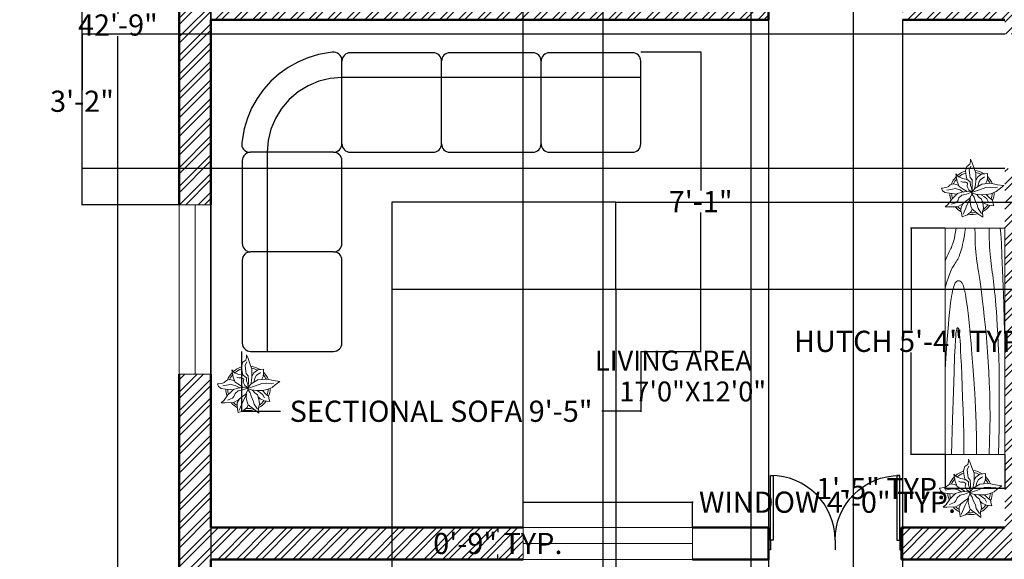
# Model space of a CAD drawing. Units: inches. Extents: x -71 to 434, y -519 to 67.
# Tile 2 of 7: x -58 to 221, y -377 to -224. Entities that reach past the tile are written whole.
import ezdxf

# ---------------------------------------------------------------- set-up
doc = ezdxf.new("R2010")
doc.units = ezdxf.units.IN
doc.header["$MEASUREMENT"] = 0
for name, color, linetype, lineweight in [('A-ANNO-DIMS', 7, 'Continuous', 18), ('A-AREA-IDEN', 7, 'Continuous', 25), ('A-WALL-PATT', 8, 'Continuous', 13), ('CAY', 94, 'Continuous', 13), ('DOOR', 3, 'Continuous', 25), ('FURNITURE', 5, 'Continuous', 18), ('WALL', 50, 'Continuous', 50), ('WINDOW', 1, 'Continuous', 18)]:
    doc.layers.add(name, color=color, linetype=linetype, lineweight=lineweight)
doc.layers.add('NOITHAT', color=21, linetype='Continuous')
doc.styles.add('ATT', font='romans.shx')
doc.styles.get("Standard").update_dxf_attribs({"font": 'arial.ttf'})
doc.dimstyles.get("Standard").update_dxf_attribs({"dimtxt": 6, "dimasz": 0.18, "dimexe": 0.18, "dimexo": 0.0625, "dimgap": 0.09, "dimtad": 0, "dimtih": 1, "dimtoh": 1, "dimdec": 0, "dimzin": 0, "dimdsep": 46, "dimlunit": 3, "dimtxsty": 'Standard', "dimcen": 0.09, "dimadec": 0, "dimazin": 0, "dimtfac": 1, "dimtdec": 0, "dimtofl": 0, "dimtmove": 0, "dimatfit": 3, "dimfxl": 1, "dimtolj": 1, "dimtzin": 0, "dimarcsym": 0})

# ---------------------------------------------------------------- blocks, each defined once
blk = doc.blocks.new('A$C74556632')
at = {"layer": 'NOITHAT'}
for p, q in [((462.2, 1788.5), (398.2, 1769.7)), ((544.2, 1802.9), (462.2, 1788.5)), ((1152.9, 1800), (652.9, 1800)), ((1752.9, 1800), (1252.9, 1800)), ((2352.9, 1800), (1852.9, 1800)), ((336.7, 1744), (278.4, 1711.6)), ((398.2, 1769.7), (336.7, 1744)), ((602.9, 1250), (602.9, 1750)), ((1202.9, 1250), (1202.9, 1750)), ((1802.9, 1250), (1802.9, 1750)), ((2402.9, 1250), (2402.9, 1750)), ((224.1, 1672.9), (174.4, 1628.5)), ((278.4, 1711.6), (224.1, 1672.9)), ((174.4, 1628.5), (130, 1578.8)), ((463.8, 1628), (398.6, 1601)), ((532.4, 1644.5), (463.8, 1628)), ((602.9, 1650), (532.4, 1644.5)), ((2402.9, 1650), (602.9, 1650)), ((130, 1578.8), (91.3, 1524.5)), ((338.3, 1564.1), (284.6, 1518.2)), ((398.6, 1601), (338.3, 1564.1)), ((91.3, 1524.5), (58.9, 1466.2)), ((284.6, 1518.2), (238.8, 1464.5)), ((58.9, 1466.2), (33.2, 1404.7)), ((238.8, 1464.5), (201.9, 1404.3)), ((33.2, 1404.7), (14.4, 1340.7)), ((201.9, 1404.3), (174.9, 1339.1)), ((14.4, 1340.7), (0, 1258.7)), ((174.9, 1339.1), (158.4, 1270.4)), ((158.4, 1270.4), (152.9, 1200)), ((552.9, 1200), (49.2, 1200)), ((152.9, 1200), (152.9, 0)), ((652.9, 1200), (1152.9, 1200)), ((677.9, 1200), (677.9, 1200)), ((1252.9, 1200), (1752.9, 1200)), ((1852.9, 1200), (2352.9, 1200)), ((2.9, 1150), (2.9, 650)), ((602.9, 650), (602.9, 1150)), ((2252.9, 900), (902.9, 900)), ((902.9, 900), (902.9, 375)), ((2252.9, 375), (2252.9, 900)), ((552.9, 600), (52.9, 600)), ((2.9, 550), (2.9, 50)), ((602.9, 50), (602.9, 550)), ((902.9, 375), (2252.9, 375)), ((52.9, 0), (552.9, 0))]:
    blk.add_line(p, q, dxfattribs=at)
for centre, start, end in [((552.9, 1753.6), 0, 99.97066), ((652.9, 1750), 90, 180), ((1152.9, 1750), 0, 90), ((1252.9, 1750), 90, 180), ((1752.9, 1750), 0, 90), ((1852.9, 1750), 90, 180), ((2352.9, 1750), 0, 90), ((49.2, 1250), 170.02934, 270), ((552.9, 1250), 270, 0), ((652.9, 1250), 180, 270), ((1152.9, 1250), 270, 0), ((1252.9, 1250), 180, 270), ((1752.9, 1250), 270, 0), ((1852.9, 1250), 180, 270), ((2352.9, 1250), 270, 0), ((52.9, 1150), 90, 180), ((552.9, 1150), 0, 90), ((52.9, 650), 180, 270), ((52.9, 550), 90, 180), ((552.9, 650), 270, 0), ((552.9, 550), 0, 90), ((52.9, 50), 180, 270), ((552.9, 50), 270, 0)]:
    blk.add_arc(centre, 50, start, end, dxfattribs=at)
blk = doc.blocks.new('*U13')
for p, q in [((0, 0), (0, -6)), ((40, 0), (40, -6))]:
    blk.add_line(p, q)
blk.add_lwpolyline([(0, 0), (0, 40), (1.75, 40), (1.75, 0)], close=True)
blk.add_arc((0, 0), 40, 0, 90)
blk = doc.blocks.new('Hutch - 19 x 72 in.')
for p, q in [((0, -19), (0, 0)), ((0, 0), (71.999994, 0)), ((71.999994, 0), (71.999994, -19)), ((71.999994, -19), (0, -19))]:
    blk.add_line(p, q)
for points in [[(26.99999, 0), (32.30411, -0.35238), (36.66731, -0.66276), (40.20336, -0.93603), (43.02603, -1.17708), (45.2491, -1.39079), (46.98632, -1.58203), (48.35147, -1.7557), (49.45833, -1.91667), (50.40388, -2.06917), (51.21809, -2.21484), (51.91414, -2.35465), (52.5052, -2.48958), (53.00447, -2.6206), (53.42512, -2.7487), (53.78035, -2.87484), (54.08333, -3), (54.34537, -3.12516), (54.57031, -3.2513), (54.76008, -3.37939), (54.91666, -3.51042), (55.04198, -3.64534), (55.13801, -3.78516), (55.2067, -3.93083), (55.24999, -4.08333), (55.26904, -4.24316), (55.26171, -4.40885), (55.22509, -4.57845), (55.15624, -4.75), (55.05224, -4.92155), (54.91015, -5.09115), (54.72704, -5.25684), (54.49999, -5.41667), (54.22493, -5.56934), (53.89322, -5.71615), (53.49511, -5.85905), (53.02083, -6), (52.4606, -6.14095), (51.80468, -6.28385), (51.04329, -6.43066), (50.16666, -6.58333), (49.16007, -6.74381), (47.98892, -6.91406), (46.61368, -7.09603), (44.99478, -7.29167), (43.09268, -7.50293), (40.86783, -7.73177), (38.28067, -7.98014), (35.29166, -8.25), (31.87654, -8.54053), (28.07226, -8.83984), (23.93107, -9.1333), (19.5052, -9.40625), (14.84692, -9.64404), (10.00846, -9.83203), (5.04207, -9.95557), (0, -10)], [(52.99999, 0), (54.87133, -0.53955), (56.39257, -1.03516), (57.61205, -1.48975), (58.57812, -1.90625), (59.3391, -2.2876), (59.94335, -2.63672), (60.4392, -2.95654), (60.87499, -3.25), (61.29247, -3.52002), (61.70702, -3.76953), (62.12743, -4.00146), (62.56249, -4.21875), (63.02099, -4.42432), (63.51171, -4.62109), (64.04345, -4.81201), (64.62499, -5), (65.26489, -5.1875), (65.9707, -5.375), (66.74975, -5.5625), (67.60937, -5.75), (68.55688, -5.9375), (69.5996, -6.125), (70.744867, -6.3125), (71.999994, -6.5)], [(61.49999, 0), (62.35961, -0.35254), (63.08007, -0.66406), (63.68627, -0.94043), (64.20312, -1.1875), (64.65551, -1.41113), (65.06835, -1.61719), (65.46655, -1.81152), (65.87499, -2), (66.31762, -2.1875), (66.81445, -2.375), (67.38452, -2.5625), (68.04687, -2.75), (68.82055, -2.9375), (69.7246, -3.125), (70.77807, -3.3125), (71.999994, -3.5)], [(0, -2), (11.2006, -2.34123), (19.90169, -2.62044), (26.43969, -2.84595), (31.15103, -3.02604), (34.37214, -3.16903), (36.43945, -3.2832), (37.68936, -3.37687), (38.45833, -3.45833), (39.02937, -3.53459), (39.472, -3.60742), (39.80232, -3.67733), (40.03645, -3.74479), (40.1905, -3.8103), (40.28059, -3.87435), (40.32283, -3.93742), (40.33333, -4), (40.32405, -4.0625), (40.29036, -4.125), (40.22346, -4.1875), (40.11458, -4.25), (39.95491, -4.3125), (39.73567, -4.375), (39.44807, -4.4375), (39.08333, -4.5), (38.62491, -4.56282), (38.02538, -4.6276), (37.22957, -4.69629), (36.18228, -4.77083), (34.82836, -4.85319), (33.11262, -4.94531), (30.97989, -5.04915), (28.37499, -5.16667), (25.27416, -5.29818), (21.77929, -5.4375), (18.02368, -5.57682), (14.14062, -5.70833), (10.26342, -5.82422), (6.52539, -5.91667), (3.05981, -5.97786), (0, -6)], [(71.999994, -9.5), (70.071934, -9.51147), (68.38801, -9.54492), (66.91113, -9.59888), (65.60416, -9.67187), (64.43001, -9.76245), (63.35156, -9.86914), (62.3317, -9.99048), (61.33333, -10.125), (60.32128, -10.27157), (59.26822, -10.43034), (58.14876, -10.60181), (56.93749, -10.78646), (55.60904, -10.98478), (54.13801, -11.19726), (52.49902, -11.4244), (50.66666, -11.66667), (48.62239, -11.92358), (46.37499, -12.19075), (43.9401, -12.46281), (41.33333, -12.73437), (38.57031, -13.00008), (35.66666, -13.25456), (32.63801, -13.49243), (29.49999, -13.70833), (26.26367, -13.89689), (22.92187, -14.05273), (19.46289, -14.17049), (15.875, -14.24479), (12.14648, -14.27026), (8.26562, -14.24154), (4.2207, -14.15324), (0, -14)], [(0, -17), (8.37556, -17.14274), (15.58268, -17.20443), (21.74194, -17.19775), (26.97395, -17.13542), (31.39933, -17.03011), (35.13866, -16.89453), (38.31257, -16.74137), (41.04166, -16.58333), (43.4322, -16.43083), (45.5332, -16.28516), (47.37931, -16.14534), (49.0052, -16.01042), (50.44555, -15.87939), (51.73502, -15.7513), (52.90828, -15.62516), (53.99999, -15.5), (55.04044, -15.37508), (56.04231, -15.25065), (57.01391, -15.1272), (57.96353, -15.00521), (58.89949, -14.88517), (59.83007, -14.76758), (60.76358, -14.65291), (61.70833, -14.54167), (62.6752, -14.43465), (63.68554, -14.33398), (64.76326, -14.24211), (65.93229, -14.16146), (67.21655, -14.09448), (68.63997, -14.04362), (70.226475, -14.01131), (71.999994, -14)], [(36.99999, -19), (42.40038, -18.8125), (47.95312, -18.625), (53.43554, -18.4375), (58.62499, -18.25), (63.29882, -18.0625), (67.23437, -17.875), (70.208978, -17.6875), (71.999994, -17.5)]]:
    blk.add_lwpolyline(points)
blk = doc.blocks.new('*D18')
at = {"layer": 'A-ANNO-DIMS', "color": 0, "lineweight": -2, "transparency": 16777216}
for p, q in [((-12.65, 30.83), (-30.15, 30.83)), ((-29.97, 30.65), (-29.97, -222.51)), ((-29.97, -481.99), (-29.97, -228.82)), ((-12.65, -482.17), (-30.15, -482.17))]:
    blk.add_line(p, q, dxfattribs=at)
at = {"layer": 'A-ANNO-DIMS', "color": 0, "transparency": 16777216}
for points in [[(-30, 30.65), (-29.94, 30.65), (-29.97, 30.83)], [(-30, -481.99), (-29.94, -481.99), (-29.97, -482.17)]]:
    blk.add_solid(points, dxfattribs=at)
at = {"layer": 'Defpoints', "color": 0, "transparency": 16777216}
for p in [(-12.59, 30.83), (-29.97, -482.17), (-12.59, -482.17)]:
    blk.add_point(p, dxfattribs=at)
at = {"layer": 'A-ANNO-DIMS', "color": 0, "transparency": 16777216, "insert": (-29.97, -225.67), "char_height": 6, "attachment_point": 5}
blk.add_mtext('\\A1;42\'-9"', dxfattribs=at)
blk = doc.blocks.new('12PPLT12')
at = {"color": 0, "linetype": 'ByBlock'}
for p, q in [((-0.05, 0.632), (-0.034, 0.694)), ((-0.034, 0.694), (-0.032, 0.751)), ((-0.032, 0.751), (-0.002, 0.689)), ((-0.002, 0.689), (0.044, 0.559)), ((-0.148, 0.486), (-0.116, 0.583)), ((-0.132, 0.367), (-0.148, 0.486)), ((-0.116, 0.583), (-0.05, 0.632)), ((-0.064, 0.51), (-0.026, 0.591)), ((-0.05, 0.38), (-0.064, 0.51)), ((0.044, 0.559), (0.09, 0.432)), ((-0.349, 0.334), (-0.362, 0.415)), ((-0.362, 0.415), (-0.303, 0.35)), ((-0.332, 0.247), (-0.349, 0.334)), ((-0.289, 0.136), (-0.332, 0.247)), ((-0.303, 0.35), (-0.208, 0.312)), ((-0.205, 0.231), (-0.251, 0.247)), ((-0.208, 0.312), (-0.105, 0.29)), ((-0.137, 0.231), (-0.205, 0.231)), ((-0.097, 0.204), (-0.137, 0.231)), ((-0.108, 0.279), (-0.132, 0.367)), ((-0.105, 0.29), (-0.037, 0.236)), ((-0.043, 0.334), (-0.05, 0.38)), ((0.003, 0.279), (-0.043, 0.334)), ((-0.037, 0.236), (-0.034, 0.158)), ((0.009, 0.169), (0.003, 0.279)), ((0.09, 0.253), (0.082, 0.174)), ((0.09, 0.432), (0.09, 0.339)), ((0.09, 0.339), (0.09, 0.253)), ((0.093, 0.282), (0.134, 0.347)), ((0.155, 0.228), (0.131, 0.13)), ((0.134, 0.347), (0.22, 0.415)), ((0.193, 0.293), (0.155, 0.228)), ((0.25, 0.328), (0.193, 0.293)), ((0.22, 0.415), (0.291, 0.421)), ((0.28, 0.353), (0.25, 0.328)), ((0.291, 0.421), (0.35, 0.429)), ((0.342, 0.266), (0.304, 0.19)), ((0.348, 0.331), (0.342, 0.266)), ((0.35, 0.429), (0.348, 0.331)), ((-0.671, 0.098), (-0.687, 0.095)), ((-0.687, 0.095), (-0.666, 0.036)), ((-0.59, 0.109), (-0.671, 0.098)), ((-0.666, 0.036), (-0.601, -0.005)), ((-0.536, 0.125), (-0.59, 0.109)), ((-0.563, 0.052), (-0.441, 0.074)), ((-0.487, 0.171), (-0.536, 0.125)), ((-0.425, 0.193), (-0.487, 0.171)), ((-0.441, 0.074), (-0.373, 0.084)), ((-0.346, 0.179), (-0.425, 0.193)), ((-0.373, 0.084), (-0.27, 0.057)), ((-0.292, 0.149), (-0.346, 0.179)), ((-0.229, 0.003), (-0.324, -0.027)), ((-0.194, 0.074), (-0.289, 0.136)), ((-0.27, 0.057), (-0.186, 0.006)), ((-0.069, 0.027), (-0.229, 0.003)), ((-0.108, 0.019), (-0.194, 0.074)), ((-0.01, 0.003), (-0.121, -0.038)), ((-0.11, 0.133), (-0.097, 0.204)), ((-0.069, 0.06), (-0.11, 0.133)), ((-0.01, 0.014), (-0.069, 0.06)), ((-0.002, 0.006), (-0.069, 0.027)), ((-0.034, 0.158), (-0.007, 0.101)), ((-0.018, -0.008), (0.074, 0.098)), ((-0.01, -0.005), (0.169, 0.055)), ((0.003, 0.017), (-0.01, 0.014)), ((0.003, -0.029), (-0.01, 0.003)), ((-0.007, 0.101), (0.003, 0.017)), ((0.006, 0.027), (0.009, 0.169)), ((0.082, 0.174), (0.061, 0.082)), ((0.074, 0.098), (0.223, 0.188)), ((0.169, 0.055), (0.315, 0.109)), ((0.223, 0.188), (0.421, 0.204)), ((0.315, 0.109), (0.413, 0.117)), ((0.413, 0.117), (0.524, 0.101)), ((0.421, 0.204), (0.573, 0.171)), ((0.545, 0.017), (0.429, -0.032)), ((0.524, 0.101), (0.578, 0.114)), ((0.613, 0.074), (0.545, 0.017)), ((0.573, 0.171), (0.716, 0.152)), ((0.716, 0.152), (0.613, 0.074)), ((-0.601, -0.005), (-0.503, -0.021)), ((-0.452, -0.152), (-0.536, -0.268)), ((-0.503, -0.021), (-0.4, -0.032)), ((-0.395, -0.094), (-0.452, -0.152)), ((-0.4, -0.032), (-0.357, -0.04)), ((-0.324, -0.027), (-0.395, -0.094)), ((-0.316, -0.187), (-0.352, -0.227)), ((-0.292, -0.122), (-0.316, -0.187)), ((-0.224, -0.059), (-0.292, -0.122)), ((-0.121, -0.038), (-0.224, -0.059)), ((-0.213, -0.263), (-0.135, -0.195)), ((-0.135, -0.195), (-0.053, -0.14)), ((-0.119, -0.304), (-0.04, -0.148)), ((-0.053, -0.14), (0.003, -0.029)), ((-0.037, -0.122), (-0.04, -0.219)), ((-0.04, -0.219), (-0.021, -0.308)), ((0.082, -0.038), (-0.018, -0.008)), ((-0.007, -0.024), (0.05, -0.105)), ((0.05, -0.105), (0.071, -0.181)), ((0.071, -0.181), (0.12, -0.282)), ((0.188, -0.054), (0.082, -0.038)), ((0.112, -0.051), (0.09, -0.043)), ((0.155, -0.108), (0.112, -0.051)), ((0.212, -0.152), (0.155, -0.108)), ((0.323, -0.051), (0.188, -0.054)), ((0.247, -0.246), (0.212, -0.152)), ((0.215, -0.062), (0.282, -0.103)), ((0.234, -0.2), (0.277, -0.241)), ((0.282, -0.103), (0.334, -0.146)), ((0.429, -0.032), (0.323, -0.051)), ((0.396, -0.124), (0.326, -0.054)), ((0.334, -0.146), (0.372, -0.217)), ((0.464, -0.176), (0.396, -0.124)), ((0.48, -0.257), (0.464, -0.176)), ((-0.536, -0.268), (-0.606, -0.328)), ((-0.606, -0.328), (-0.522, -0.328)), ((-0.522, -0.328), (-0.324, -0.325)), ((-0.387, -0.241), (-0.465, -0.268)), ((-0.352, -0.227), (-0.387, -0.241)), ((-0.324, -0.325), (-0.213, -0.263)), ((-0.244, -0.33), (-0.247, -0.406)), ((-0.247, -0.406), (-0.233, -0.471)), ((-0.193, -0.236), (-0.244, -0.33)), ((-0.199, -0.494), (-0.139, -0.358)), ((-0.139, -0.358), (-0.119, -0.304)), ((-0.102, -0.503), (-0.017, -0.432)), ((-0.021, -0.308), (0.006, -0.376)), ((-0.017, -0.432), (0.003, -0.378)), ((0.006, -0.376), (0.074, -0.428)), ((0.074, -0.428), (0.158, -0.496)), ((0.12, -0.282), (0.139, -0.363)), ((0.139, -0.363), (0.212, -0.474)), ((0.236, -0.444), (0.261, -0.349)), ((0.261, -0.349), (0.247, -0.246)), ((0.277, -0.241), (0.372, -0.287)), ((0.372, -0.287), (0.494, -0.301)), ((0.494, -0.301), (0.48, -0.257)), ((-0.233, -0.471), (-0.222, -0.551)), ((-0.222, -0.551), (-0.148, -0.522)), ((-0.148, -0.522), (-0.102, -0.503)), ((0.158, -0.496), (0.242, -0.561)), ((0.242, -0.561), (0.236, -0.444))]:
    blk.add_line(p, q, dxfattribs=at)
for radius, start, end in [(0.5, 107.123, 130.9816), (0.5, 56.9563, 82.295), (0.458, 62.6899, 79.5345), (0.5, 134.8021, 159.1804), (0.458, 138.4756, 155.3347), (0.458, 107.9864, 130.5771), (0.458, 26.2761, 41.1349), (0.5, 22.9768, 45.8473), (0.5, 182.503, 200.4563), (0.458, 183.2699, 197.4002), (0.458, 340.6559, 357.5057), (0.5, 338.5862, 359.7442), (0.5, 220.6606, 241.3393), (0.458, 225.0835, 237.5023), (0.5, 298.3455, 324.4541), (0.458, 303.3868, 322.0756), (0.5, 259.7038, 286.1281), (0.458, 264.1886, 282.4028)]:
    blk.add_arc((0, 0), radius, start, end, dxfattribs=at)
at = {"color": 0, "linetype": 'ByBlock', "style": 'ATT'}
for tag, p, flags in [('ITEM', (-1, -3.25), 3), ('ROOM_NUMBER', (-1, -4.583), 1)]:
    blk.add_attdef(tag, p, '', height=1, dxfattribs=dict(at, flags=flags))
blk = doc.blocks.new('WIN-48x9')
blk.add_line((0, 4.5), (48, 4.5))
blk.add_lwpolyline([(0, 0), (48, 0), (48, 9), (0, 9)], close=True)
blk = doc.blocks.new('*D26')
at = {"layer": 'A-ANNO-DIMS', "color": 0, "lineweight": -2, "transparency": 16777216}
for p, q in [((84.91, -368.1), (84.91, -360.79)), ((85.09, -360.97), (132.73, -360.97)), ((132.91, -368.1), (132.91, -360.79)), ((132.91, -360.97), (133.09, -360.97))]:
    blk.add_line(p, q, dxfattribs=at)
at = {"layer": 'A-ANNO-DIMS', "color": 0, "transparency": 16777216}
for points in [[(85.09, -360.94), (85.09, -361), (84.91, -360.97)], [(132.73, -360.94), (132.73, -361), (132.91, -360.97)]]:
    blk.add_solid(points, dxfattribs=at)
at = {"layer": 'Defpoints', "color": 0, "transparency": 16777216}
for p in [(132.91, -360.97), (84.91, -368.17), (132.91, -368.17)]:
    blk.add_point(p, dxfattribs=at)
at = {"layer": 'A-ANNO-DIMS', "color": 0, "transparency": 16777216, "insert": (171.14, -360.97), "char_height": 6, "attachment_point": 5}
blk.add_mtext('\\A1;WINDOW 4\'-0" TYP.', dxfattribs=at)
blk = doc.blocks.new('*D27')
at = {"layer": 'A-ANNO-DIMS', "color": 0, "lineweight": -2, "transparency": 16777216}
for p, q in [((84.85, -368.17), (77.53, -368.17)), ((77.71, -368.35), (77.71, -369.51)), ((77.71, -376.99), (77.71, -375.82)), ((84.85, -377.17), (77.53, -377.17))]:
    blk.add_line(p, q, dxfattribs=at)
at = {"layer": 'A-ANNO-DIMS', "color": 0, "transparency": 16777216}
for points in [[(77.68, -368.35), (77.74, -368.35), (77.71, -368.17)], [(77.68, -376.99), (77.74, -376.99), (77.71, -377.17)]]:
    blk.add_solid(points, dxfattribs=at)
at = {"layer": 'Defpoints', "color": 0, "transparency": 16777216}
for p in [(77.71, -368.17), (84.91, -368.17), (84.91, -377.17)]:
    blk.add_point(p, dxfattribs=at)
at = {"layer": 'A-ANNO-DIMS', "color": 0, "transparency": 16777216, "insert": (77.71, -372.67), "char_height": 6, "attachment_point": 5}
blk.add_mtext('\\A1;0\'-9" TYP.', dxfattribs=at)
blk = doc.blocks.new('*D32')
at = {"layer": 'A-ANNO-DIMS', "color": 0, "lineweight": -2, "transparency": 16777216}
for p, q in [((204.4, -283.25), (194.65, -283.25)), ((194.83, -283.43), (194.83, -312.16)), ((194.83, -347.28), (194.83, -318.55)), ((204.4, -347.46), (194.65, -347.46))]:
    blk.add_line(p, q, dxfattribs=at)
at = {"layer": 'A-ANNO-DIMS', "color": 0, "transparency": 16777216}
for points in [[(194.8, -283.43), (194.86, -283.43), (194.83, -283.25)], [(194.8, -347.28), (194.86, -347.28), (194.83, -347.46)]]:
    blk.add_solid(points, dxfattribs=at)
at = {"layer": 'Defpoints', "color": 0, "transparency": 16777216}
for p in [(194.83, -283.25), (204.46, -283.25), (204.46, -347.46)]:
    blk.add_point(p, dxfattribs=at)
at = {"layer": 'A-ANNO-DIMS', "color": 0, "transparency": 16777216, "insert": (194.83, -315.36), "char_height": 6, "attachment_point": 5}
blk.add_mtext('\\A1;HUTCH 5\'-4" TYP.', dxfattribs=at)
blk = doc.blocks.new('*D33')
at = {"layer": 'A-ANNO-DIMS', "color": 0, "lineweight": -2, "transparency": 16777216}
for p, q in [((204.46, -347.52), (204.46, -357.27)), ((221.41, -347.52), (221.41, -357.27)), ((204.46, -357.09), (204.28, -357.09)), ((221.23, -357.09), (204.64, -357.09))]:
    blk.add_line(p, q, dxfattribs=at)
at = {"layer": 'A-ANNO-DIMS', "color": 0, "transparency": 16777216}
for points in [[(204.64, -357.06), (204.64, -357.12), (204.46, -357.09)], [(221.23, -357.06), (221.23, -357.12), (221.41, -357.09)]]:
    blk.add_solid(points, dxfattribs=at)
at = {"layer": 'Defpoints', "color": 0, "transparency": 16777216}
for p in [(204.46, -347.46), (221.41, -347.46), (204.46, -357.09)]:
    blk.add_point(p, dxfattribs=at)
at = {"layer": 'A-ANNO-DIMS', "color": 0, "transparency": 16777216, "insert": (186.19, -357.09), "char_height": 6, "attachment_point": 5}
blk.add_mtext('\\A1;1\'-5" TYP.', dxfattribs=at)
blk = doc.blocks.new('*D40')
at = {"layer": 'A-ANNO-DIMS', "color": 0, "lineweight": -2, "transparency": 16777216}
for p, q in [((5.04, -318.28), (5.04, -335.37)), ((118.21, -318.28), (118.21, -335.37)), ((5.22, -335.19), (16.08, -335.19)), ((118.03, -335.19), (107.17, -335.19))]:
    blk.add_line(p, q, dxfattribs=at)
at = {"layer": 'A-ANNO-DIMS', "color": 0, "transparency": 16777216}
for points in [[(5.22, -335.16), (5.22, -335.22), (5.04, -335.19)], [(118.03, -335.16), (118.03, -335.22), (118.21, -335.19)]]:
    blk.add_solid(points, dxfattribs=at)
at = {"layer": 'Defpoints', "color": 0, "transparency": 16777216}
for p in [(5.04, -318.22), (118.21, -318.22), (118.21, -335.19)]:
    blk.add_point(p, dxfattribs=at)
at = {"layer": 'A-ANNO-DIMS', "color": 0, "transparency": 16777216, "insert": (61.62, -335.19), "char_height": 6, "attachment_point": 5}
blk.add_mtext('\\A1;SECTIONAL SOFA 9\'-5"', dxfattribs=at)
blk = doc.blocks.new('*D41')
at = {"layer": 'A-ANNO-DIMS', "color": 0, "lineweight": -2, "transparency": 16777216}
for p, q in [((118.27, -233.27), (135.37, -233.27)), ((135.19, -233.45), (135.19, -272.64)), ((135.19, -318.04), (135.19, -278.85)), ((118.27, -318.22), (135.37, -318.22))]:
    blk.add_line(p, q, dxfattribs=at)
at = {"layer": 'A-ANNO-DIMS', "color": 0, "transparency": 16777216}
for points in [[(135.16, -233.45), (135.22, -233.45), (135.19, -233.27)], [(135.16, -318.04), (135.22, -318.04), (135.19, -318.22)]]:
    blk.add_solid(points, dxfattribs=at)
at = {"layer": 'Defpoints', "color": 0, "transparency": 16777216}
for p in [(118.21, -233.27), (135.19, -233.27), (118.21, -318.22)]:
    blk.add_point(p, dxfattribs=at)
at = {"layer": 'A-ANNO-DIMS', "color": 0, "transparency": 16777216, "insert": (135.19, -275.74), "char_height": 6, "attachment_point": 5}
blk.add_mtext('\\A1;7\'-1"', dxfattribs=at)
blk = doc.blocks.new('*D45')
at = {"layer": 'A-ANNO-DIMS', "color": 0, "lineweight": -2, "transparency": 16777216}
for p, q in [((-12.65, -68.17), (-40.32, -68.17)), ((-40.14, -68.35), (-40.14, -169.22)), ((-40.14, -276.49), (-40.14, -175.61)), ((-12.65, -276.67), (-40.32, -276.67))]:
    blk.add_line(p, q, dxfattribs=at)
at = {"layer": 'A-ANNO-DIMS', "color": 0, "transparency": 16777216}
for points in [[(-40.17, -68.35), (-40.11, -68.35), (-40.14, -68.17)], [(-40.17, -276.49), (-40.11, -276.49), (-40.14, -276.67)]]:
    blk.add_solid(points, dxfattribs=at)
at = {"layer": 'Defpoints', "color": 0, "transparency": 16777216}
for p in [(-12.59, -68.17), (-40.14, -276.67), (-12.59, -276.67)]:
    blk.add_point(p, dxfattribs=at)
at = {"layer": 'A-ANNO-DIMS', "color": 0, "transparency": 16777216, "insert": (-40.14, -172.42), "char_height": 6, "attachment_point": 5}
blk.add_mtext('\\A1;17\'-4 1/2"', dxfattribs=at)
blk = doc.blocks.new('*D46')
at = {"layer": 'A-ANNO-DIMS', "color": 0, "lineweight": -2, "transparency": 16777216}
for p, q in [((-3.59, -368.1), (-3.59, 58.56)), ((-3.41, 58.38), (25.63, 58.38)), ((84.73, 58.38), (55.69, 58.38)), ((84.91, -368.1), (84.91, 58.56))]:
    blk.add_line(p, q, dxfattribs=at)
at = {"layer": 'A-ANNO-DIMS', "color": 0, "transparency": 16777216}
for points in [[(-3.41, 58.41), (-3.41, 58.35), (-3.59, 58.38)], [(84.73, 58.41), (84.73, 58.35), (84.91, 58.38)]]:
    blk.add_solid(points, dxfattribs=at)
at = {"layer": 'Defpoints', "color": 0, "transparency": 16777216}
for p in [(84.91, 58.38), (-3.59, -368.17), (84.91, -368.17)]:
    blk.add_point(p, dxfattribs=at)
at = {"layer": 'A-ANNO-DIMS', "color": 0, "transparency": 16777216, "insert": (40.66, 58.38), "char_height": 6, "attachment_point": 5}
blk.add_mtext('\\A1;7\'-4 1/2"', dxfattribs=at)
blk = doc.blocks.new('*D56')
at = {"layer": 'A-ANNO-DIMS', "color": 0, "lineweight": -2, "transparency": 16777216}
for p, q in [((154.41, -71.23), (154.41, -509.9)), ((178.41, -71.23), (178.41, -509.9)), ((154.59, -509.72), (158.29, -509.72)), ((178.23, -509.72), (174.52, -509.72))]:
    blk.add_line(p, q, dxfattribs=at)
at = {"layer": 'A-ANNO-DIMS', "color": 0, "transparency": 16777216}
for points in [[(154.59, -509.69), (154.59, -509.75), (154.41, -509.72)], [(178.23, -509.69), (178.23, -509.75), (178.41, -509.72)]]:
    blk.add_solid(points, dxfattribs=at)
at = {"layer": 'Defpoints', "color": 0, "transparency": 16777216}
for p in [(154.41, -71.17), (178.41, -71.17), (178.41, -509.72)]:
    blk.add_point(p, dxfattribs=at)
at = {"layer": 'A-ANNO-DIMS', "color": 0, "transparency": 16777216, "insert": (166.41, -509.72), "char_height": 6, "attachment_point": 5}
blk.add_mtext('\\A1;2\'-0"', dxfattribs=at)
blk = doc.blocks.new('*D58')
at = {"layer": 'A-ANNO-DIMS', "color": 0, "lineweight": -2, "transparency": 16777216}
for p, q in [((221.35, -228.23), (-40.32, -228.23)), ((-40.14, -228.41), (-40.14, -244.13)), ((-40.14, -266.16), (-40.14, -250.44)), ((221.35, -266.34), (-40.32, -266.34))]:
    blk.add_line(p, q, dxfattribs=at)
at = {"layer": 'A-ANNO-DIMS', "color": 0, "transparency": 16777216}
for points in [[(-40.17, -228.41), (-40.11, -228.41), (-40.14, -228.23)], [(-40.17, -266.16), (-40.11, -266.16), (-40.14, -266.34)]]:
    blk.add_solid(points, dxfattribs=at)
at = {"layer": 'Defpoints', "color": 0, "transparency": 16777216}
for p in [(221.41, -228.23), (-40.14, -266.34), (221.41, -266.34)]:
    blk.add_point(p, dxfattribs=at)
at = {"layer": 'A-ANNO-DIMS', "color": 0, "transparency": 16777216, "insert": (-40.14, -247.29), "char_height": 6, "attachment_point": 5}
blk.add_mtext('\\A1;3\'-2"', dxfattribs=at)
blk = doc.blocks.new('*D62')
at = {"layer": 'A-ANNO-DIMS', "color": 0, "lineweight": -2, "transparency": 16777216}
for p, q in [((149.41, -71.23), (149.41, -509.9)), ((154.41, -71.23), (154.41, -509.9)), ((149.59, -509.72), (154.23, -509.72)), ((154.41, -509.72), (154.59, -509.72))]:
    blk.add_line(p, q, dxfattribs=at)
at = {"layer": 'A-ANNO-DIMS', "color": 0, "transparency": 16777216}
for points in [[(149.59, -509.69), (149.59, -509.75), (149.41, -509.72)], [(154.23, -509.69), (154.23, -509.75), (154.41, -509.72)]]:
    blk.add_solid(points, dxfattribs=at)
at = {"layer": 'Defpoints', "color": 0, "transparency": 16777216}
for p in [(149.41, -71.17), (154.41, -71.17), (154.41, -509.72)]:
    blk.add_point(p, dxfattribs=at)
at = {"layer": 'A-ANNO-DIMS', "color": 0, "transparency": 16777216, "insert": (162.65, -509.72), "char_height": 6, "attachment_point": 5}
blk.add_mtext('\\A1;0\'-5"', dxfattribs=at)
blk = doc.blocks.new('*D66')
at = {"layer": 'A-ANNO-DIMS', "color": 0, "lineweight": -2, "transparency": 16777216}
for p, q in [((-3.59, -119.23), (-3.59, -509.9)), ((107.49, -119.23), (107.49, -509.9)), ((-3.41, -509.72), (43.89, -509.72)), ((107.31, -509.72), (60.02, -509.72))]:
    blk.add_line(p, q, dxfattribs=at)
at = {"layer": 'A-ANNO-DIMS', "color": 0, "transparency": 16777216}
for points in [[(-3.41, -509.69), (-3.41, -509.75), (-3.59, -509.72)], [(107.31, -509.69), (107.31, -509.75), (107.49, -509.72)]]:
    blk.add_solid(points, dxfattribs=at)
at = {"layer": 'Defpoints', "color": 0, "transparency": 16777216}
for p in [(-3.59, -119.17), (107.49, -119.17), (107.49, -509.72)]:
    blk.add_point(p, dxfattribs=at)
at = {"layer": 'A-ANNO-DIMS', "color": 0, "transparency": 16777216, "insert": (51.95, -509.72), "char_height": 6, "attachment_point": 5}
blk.add_mtext('\\A1;9\'-3"', dxfattribs=at)
blk = doc.blocks.new('*D70')
at = {"layer": 'A-ANNO-DIMS', "color": 0, "lineweight": -2, "transparency": 16777216}
for p, q in [((154.41, -224.23), (154.41, -509.9)), ((192.42, -224.23), (192.42, -509.9)), ((154.59, -509.72), (165.35, -509.72)), ((192.24, -509.72), (181.47, -509.72))]:
    blk.add_line(p, q, dxfattribs=at)
at = {"layer": 'A-ANNO-DIMS', "color": 0, "transparency": 16777216}
for points in [[(154.59, -509.69), (154.59, -509.75), (154.41, -509.72)], [(192.24, -509.69), (192.24, -509.75), (192.42, -509.72)]]:
    blk.add_solid(points, dxfattribs=at)
at = {"layer": 'Defpoints', "color": 0, "transparency": 16777216}
for p in [(154.41, -224.17), (192.42, -224.17), (192.42, -509.72)]:
    blk.add_point(p, dxfattribs=at)
at = {"layer": 'A-ANNO-DIMS', "color": 0, "transparency": 16777216, "insert": (173.41, -509.72), "char_height": 6, "attachment_point": 5}
blk.add_mtext('\\A1;3\'-2"', dxfattribs=at)
blk = doc.blocks.new('*D71')
at = {"layer": 'A-ANNO-DIMS', "color": 0, "lineweight": -2, "transparency": 16777216}
for p, q in [((47.64, -300.64), (47.64, -509.9)), ((111.15, -300.64), (111.15, -509.9)), ((47.82, -509.72), (64.34, -509.72)), ((110.97, -509.72), (94.45, -509.72))]:
    blk.add_line(p, q, dxfattribs=at)
at = {"layer": 'A-ANNO-DIMS', "color": 0, "transparency": 16777216}
for points in [[(47.82, -509.69), (47.82, -509.75), (47.64, -509.72)], [(110.97, -509.69), (110.97, -509.75), (111.15, -509.72)]]:
    blk.add_solid(points, dxfattribs=at)
at = {"layer": 'Defpoints', "color": 0, "transparency": 16777216}
for p in [(47.64, -300.57), (111.15, -300.57), (111.15, -509.72)]:
    blk.add_point(p, dxfattribs=at)
at = {"layer": 'A-ANNO-DIMS', "color": 0, "transparency": 16777216, "insert": (79.4, -509.72), "char_height": 6, "attachment_point": 5}
blk.add_mtext('\\A1;5\'-3 1/2"', dxfattribs=at)
blk = doc.blocks.new('*D72')
at = {"layer": 'A-ANNO-DIMS', "color": 0, "lineweight": -2, "transparency": 16777216}
for p, q in [((111.22, -275.87), (411.14, -275.87)), ((410.96, -276.05), (410.96, -285.03)), ((410.96, -300.39), (410.96, -291.41)), ((111.22, -300.57), (411.14, -300.57))]:
    blk.add_line(p, q, dxfattribs=at)
at = {"layer": 'A-ANNO-DIMS', "color": 0, "transparency": 16777216}
for points in [[(410.93, -276.05), (410.99, -276.05), (410.96, -275.87)], [(410.93, -300.39), (410.99, -300.39), (410.96, -300.57)]]:
    blk.add_solid(points, dxfattribs=at)
at = {"layer": 'Defpoints', "color": 0, "transparency": 16777216}
for p in [(111.15, -275.87), (111.15, -300.57), (410.96, -300.57)]:
    blk.add_point(p, dxfattribs=at)
at = {"layer": 'A-ANNO-DIMS', "color": 0, "transparency": 16777216, "insert": (410.96, -288.22), "char_height": 6, "attachment_point": 5}
blk.add_mtext('\\A1;2\'-0 1/2"', dxfattribs=at)

msp = doc.modelspace()

# ---------------------------------------------------------------- hatches: boundary and pattern name
at = {"layer": 'A-WALL-PATT'}
h = msp.add_hatch(dxfattribs=at)
h.set_pattern_fill('ANSI32', color=256, scale=10)
h.set_pattern_definition([(45, (-213.138, 0), (-2.65165, 2.65165), []), (45, (-211.37, 0), (-2.65165, 2.65165), [])])
h.paths.add_polyline_path([(383.41, 30.83), (230.41, 30.83), (149.41, 30.83), (-12.59, 30.83), (-12.59, -20.17), (-3.59, -20.17), (-3.59, 21.83), (140.41, 21.83), (140.41, 15.83), (149.41, 15.83), (149.41, 21.83), (221.41, 21.83), (221.41, 15.83), (230.41, 15.83), (230.41, 21.83), (374.41, 21.83), (374.41, -110.17), (369.41, -110.17), (369.41, -119.17), (374.41, -119.17), (374.41, -215.17), (320.41, -215.17), (320.41, -119.17), (345.41, -119.17), (345.41, -110.17), (221.41, -110.17), (221.41, -119.17), (311.41, -119.17), (311.41, -215.17), (192.42, -215.17), (192.42, -224.17), (221.41, -224.17), (221.41, -228.23), (230.41, -228.23), (230.41, -224.17), (374.41, -224.17), (374.41, -368.17), (230.41, -368.17), (230.41, -266.34), (221.41, -266.34), (221.41, -368.17), (192.08, -368.17), (192.08, -377.17), (230.41, -377.17), (374.41, -377.17), (374.41, -473.17), (230.41, -473.17), (212.41, -473.17), (212.41, -482.17), (383.41, -482.17), (383.41, -377.17), (383.41, -224.17), (383.41, -119.17)])
h.paths.add_polyline_path([(149.41, -110.17), (-3.59, -110.17), (-3.59, -68.17), (-12.59, -68.17), (-12.59, -276.67), (-3.59, -276.67), (-3.59, -224.17), (154.41, -224.17), (154.41, -215.17), (149.41, -215.17), (149.41, -154.17), (140.41, -154.17), (140.41, -215.17), (-3.59, -215.17), (-3.59, -119.17), (19.82, -119.17), (140.41, -119.17), (140.41, -124.17), (149.41, -124.17)])
h.paths.add_polyline_path([(84.91, -368.17), (-3.59, -368.17), (-3.59, -324.67), (-12.59, -324.67), (-12.59, -377.17), (-12.59, -401.17), (-3.59, -401.17), (-3.59, -377.17), (84.91, -377.17)], flags=17)
h.paths.add_polyline_path([(1.41, -473.17), (-3.59, -473.17), (-3.59, -468.17), (-12.59, -468.17), (-12.59, -482.17), (1.41, -482.17)], flags=17)

# ---------------------------------------------------------------- linework, layer by layer
at = {"layer": 'DOOR'}
for p, q in [((154.96, -374.44), (154.41, -374.44)), ((191.6, -374.44), (192.08, -374.44))]:
    msp.add_line(p, q, dxfattribs=at)
at = {"layer": 'WALL'}
for p, q in [((-12.59, -68.17), (-12.59, -276.67)), ((154.41, -224.17), (154.41, -215.17)), ((-3.59, -224.17), (154.41, -224.17)), ((-3.59, -224.17), (-3.59, -276.67)), ((192.42, -224.17), (221.41, -224.17)), ((-12.59, -324.67), (-12.59, -377.17)), ((-3.59, -324.67), (-3.59, -368.17)), ((-3.59, -368.17), (84.91, -368.17)), ((132.91, -368.17), (154.41, -368.17)), ((154.41, -368.17), (154.41, -377.17)), ((192.08, -368.17), (192.08, -377.17)), ((192.08, -368.17), (221.41, -368.17)), ((-12.59, -377.17), (-12.59, -401.17)), ((-3.59, -377.17), (84.91, -377.17)), ((-3.59, -377.17), (-3.59, -401.17)), ((132.91, -377.17), (149.41, -377.17)), ((149.41, -377.17), (154.41, -377.17)), ((192.08, -377.17), (230.41, -377.17))]:
    msp.add_line(p, q, dxfattribs=at)

# ---------------------------------------------------------------- block references
at = {"layer": 'CAY', "xscale": 12.58515090877727, "yscale": 12.58515090877727, "zscale": 12.58515090877727}
for p in [(212.06, -273.13), (6.9, -328.65), (211.52, -358.21)]:
    msp.add_blockref('12PPLT12', p, dxfattribs=at)
at = {"layer": 'DOOR', "yscale": 0.4579749947461901, "zscale": 0.4579749947461901}
for p, xscale in [((154.96, -371.69), 0.4579749947461901), ((191.6, -371.69), -0.4579749947461901)]:
    msp.add_blockref('*U13', p, dxfattribs=dict(at, xscale=xscale))
at = {"layer": 'FURNITURE', "xscale": 0.0470482243741732, "yscale": 0.0470482243741732, "zscale": 0.0470482243741732}
msp.add_blockref('A$C74556632', (5.16, -318.22), dxfattribs=at)
at = {"layer": 'FURNITURE', "xscale": 0.8917373781469976, "yscale": 0.8917373781469976, "zscale": 0.8917373781469976, "rotation": 90}
msp.add_blockref('Hutch - 19 x 72 in.', (204.46, -347.46), dxfattribs=at)
at = {"layer": 'WINDOW', "rotation": 270}
msp.add_blockref('WIN-48x9', (-12.59, -276.67), dxfattribs=at)
at = {"layer": 'WINDOW'}
msp.add_blockref('WIN-48x9', (84.91, -377.17), dxfattribs=at)

# ---------------------------------------------------------------- texts
at = {"layer": 'A-AREA-IDEN'}
for s, p in [('LIVING AREA', (105.21, -323.64)), ('17\'0"X12\'0"', (112.12, -332.4))]:
    msp.add_text(s, height=5.6432, dxfattribs=at).set_placement(p)

# ---------------------------------------------------------------- dimensions: what is measured, and where the dimension line sits
at = {"layer": 'A-ANNO-DIMS'}
for base, p1, p2, picture, middle in [((84.91, 58.38), (-3.59, -368.17), (84.91, -368.17), '*D46', (40.66, 58.38)), ((154.41, -509.72), (149.41, -71.17), (154.41, -71.17), '*D62', (162.65, -509.72)), ((178.41, -509.72), (154.41, -71.17), (178.41, -71.17), '*D56', (166.41, -509.72)), ((107.49, -509.72), (-3.59, -119.17), (107.49, -119.17), '*D66', (51.95, -509.72)), ((192.42, -509.72), (154.41, -224.17), (192.42, -224.17), '*D70', (173.41, -509.72)), ((111.15, -509.72), (47.64, -300.57), (111.15, -300.57), '*D71', (79.4, -509.72))]:
    dim = msp.add_linear_dim(base=base, p1=p1, p2=p2, dimstyle='Standard', override={"dimdec": 1, "dimlfac": 1, "dimrnd": 0, "dimzin": 1, "dimdsep": 46, "dimlunit": 4, "dimfrac": 2}, dxfattribs=at)
    dim.commit()
    dim.dimension.update_dxf_attribs({"geometry": picture, "text_midpoint": middle})
for base, p1, p2, override, picture, middle in [((-29.97, -482.17), (-12.59, 30.83), (-12.59, -482.17), {"dimclrd": 0, "dimclre": 0, "dimclrt": 0}, '*D18', (-29.97, -225.67)), ((-40.14, -276.67), (-12.59, -68.17), (-12.59, -276.67), {"dimdec": 1, "dimlfac": 1, "dimrnd": 0, "dimzin": 1, "dimdsep": 46, "dimlunit": 4, "dimfrac": 2}, '*D45', (-40.14, -172.42)), ((-40.14, -266.34), (221.41, -228.23), (221.41, -266.34), {"dimdec": 1, "dimlfac": 1, "dimrnd": 0, "dimzin": 1, "dimdsep": 46, "dimlunit": 4, "dimfrac": 2}, '*D58', (-40.14, -247.29)), ((135.1862, -233.2733), (118.2105, -318.2157), (118.2105, -233.2733), {"dimdec": 1, "dimlfac": 1, "dimrnd": 0, "dimzin": 1, "dimdsep": 46, "dimlunit": 4, "dimfrac": 2}, '*D41', (135.1862, -275.7445)), ((410.96, -300.57), (111.15, -275.87), (111.15, -300.57), {"dimdec": 1, "dimlfac": 1, "dimrnd": 0, "dimzin": 1, "dimdsep": 46, "dimlunit": 4, "dimfrac": 2}, '*D72', (410.96, -288.22))]:
    dim = msp.add_linear_dim(base=base, p1=p1, p2=p2, angle=90, dimstyle='Standard', override=override, dxfattribs=at)
    dim.commit()
    dim.dimension.update_dxf_attribs({"geometry": picture, "text_midpoint": middle})
for base, p1, p2, angle, text, picture, middle in [((194.83, -283.25), (204.46, -347.46), (204.46, -283.25), 90, 'HUTCH <> TYP.', '*D32', (194.83, -315.36)), ((204.4648, -357.0885), (221.4078, -347.4577), (204.4648, -347.4577), 180, '<> TYP.', '*D33', (186.1907, -357.0885)), ((77.71, -368.17), (84.91, -377.17), (84.91, -368.17), 90, '<> TYP.', '*D27', (77.71, -372.67))]:
    dim = msp.add_linear_dim(base=base, p1=p1, p2=p2, angle=angle, text=text, dimstyle='Standard', override={"dimdec": 1, "dimlfac": 1, "dimrnd": 0, "dimzin": 1, "dimdsep": 46, "dimlunit": 4, "dimfrac": 2}, dxfattribs=at)
    dim.commit()
    dim.dimension.update_dxf_attribs({"geometry": picture, "text_midpoint": middle})
for base, p1, p2, text, picture, middle in [((118.21, -335.19), (5.04, -318.22), (118.21, -318.22), 'SECTIONAL SOFA <>', '*D40', (61.62, -335.19)), ((132.91, -360.97), (84.91, -368.17), (132.91, -368.17), 'WINDOW <> TYP.', '*D26', (171.14, -360.97))]:
    dim = msp.add_linear_dim(base=base, p1=p1, p2=p2, text=text, dimstyle='Standard', override={"dimdec": 1, "dimlfac": 1, "dimrnd": 0, "dimzin": 1, "dimdsep": 46, "dimlunit": 4, "dimfrac": 2}, dxfattribs=at)
    dim.commit()
    dim.dimension.update_dxf_attribs({"geometry": picture, "text_midpoint": middle})

doc.saveas('drawing.dxf')
